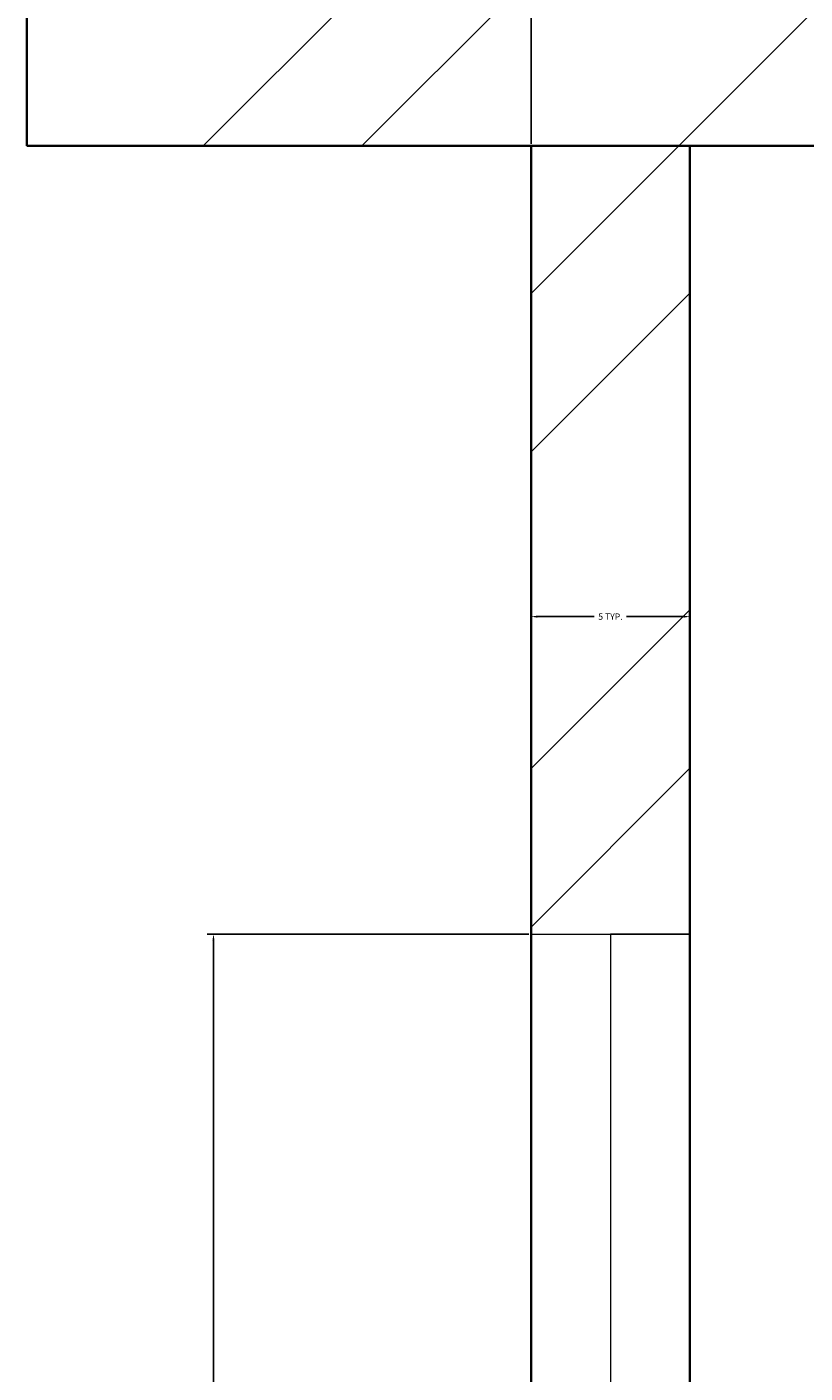
# Model space of a CAD drawing. Units: inches. Extents: x 1962 to 2771, y 1245 to 2660.
# Tile 28 of 114: x 2072 to 2094, y 1894 to 1932. Entities that reach past the tile are written whole.
import ezdxf

# ---------------------------------------------------------------- set-up
doc = ezdxf.new("R2010")
doc.units = ezdxf.units.IN
for name, color, linetype, lineweight in [('A-ANNO-DIMS', 2, 'Continuous', 18), ('A-GLAZ', 4, 'Continuous', 18), ('A-WALL', 7, 'Continuous', 35), ('A-WALL-PATT', 252, 'Continuous', 13)]:
    doc.layers.add(name, color=color, linetype=linetype, lineweight=lineweight)
doc.styles.get("Standard").update_dxf_attribs({"font": 'arial.ttf'})
doc.dimstyles.get("Standard").update_dxf_attribs({"dimtxt": 0.18, "dimasz": 0.18, "dimexe": 0.18, "dimexo": 0.0625, "dimgap": 0.09, "dimtad": 0, "dimtih": 1, "dimtoh": 1, "dimdec": 4, "dimzin": 0, "dimdsep": 46, "dimtxsty": 'Standard', "dimcen": 0.09, "dimadec": 0, "dimazin": 0, "dimtfac": 1, "dimtdec": 4, "dimtofl": 0, "dimtmove": 0, "dimatfit": 3, "dimfxl": 1, "dimtolj": 1, "dimtzin": 0, "dimarcsym": 0})

# ---------------------------------------------------------------- blocks, each defined once
blk = doc.blocks.new('WIN-60IN-A')
for p, q in [((0, 60), (4.5, 60)), ((4.5, 60), (2.25, 60)), ((2.25, 60), (2.25, 0))]:
    blk.add_line(p, q)
blk = doc.blocks.new('*D22')
at = {"layer": 'A-ANNO-DIMS', "color": 0, "lineweight": -2, "transparency": 16777216}
for p, q in [((2086.245, 1906.501), (2077.127, 1906.501)), ((2077.307, 1906.321), (2077.307, 1876.683)), ((2077.307, 1846.681), (2077.307, 1876.319)), ((2086.245, 1846.501), (2077.127, 1846.501))]:
    blk.add_line(p, q, dxfattribs=at)
at = {"layer": 'A-ANNO-DIMS', "color": 0, "transparency": 16777216}
for points in [[(2077.277, 1906.321), (2077.337, 1906.321), (2077.307, 1906.501)], [(2077.277, 1846.681), (2077.337, 1846.681), (2077.307, 1846.501)]]:
    blk.add_solid(points, dxfattribs=at)
at = {"layer": 'Defpoints', "color": 0, "transparency": 16777216}
for p in [(2077.307, 1906.501), (2086.307, 1906.501), (2086.307, 1846.501)]:
    blk.add_point(p, dxfattribs=at)
at = {"layer": 'A-ANNO-DIMS', "color": 0, "transparency": 16777216, "insert": (2077.307, 1876.501), "char_height": 0.18, "attachment_point": 5}
blk.add_mtext('\\A1;W3A 60 TYP.', dxfattribs=at)
blk = doc.blocks.new('*D23')
at = {"layer": 'A-ANNO-DIMS', "color": 0, "lineweight": -2, "transparency": 16777216}
for p, q in [((2086.307, 1906.564), (2086.307, 1915.681)), ((2086.487, 1915.501), (2088.099, 1915.501)), ((2090.627, 1915.501), (2089.016, 1915.501)), ((2090.807, 1906.564), (2090.807, 1915.681))]:
    blk.add_line(p, q, dxfattribs=at)
at = {"layer": 'A-ANNO-DIMS', "color": 0, "transparency": 16777216}
for points in [[(2086.487, 1915.531), (2086.487, 1915.471), (2086.307, 1915.501)], [(2090.627, 1915.531), (2090.627, 1915.471), (2090.807, 1915.501)]]:
    blk.add_solid(points, dxfattribs=at)
at = {"layer": 'Defpoints', "color": 0, "transparency": 16777216}
for p in [(2090.807, 1915.501), (2086.307, 1906.501), (2090.807, 1906.501)]:
    blk.add_point(p, dxfattribs=at)
at = {"layer": 'A-ANNO-DIMS', "color": 0, "transparency": 16777216, "insert": (2088.557, 1915.501), "char_height": 0.18, "attachment_point": 5}
blk.add_mtext('\\A1;5 TYP.', dxfattribs=at)
blk = doc.blocks.new('*D41')
at = {"layer": 'A-ANNO-DIMS', "color": 0, "lineweight": -2, "transparency": 16777216}
for p, q in [((2072.02, 1928.906), (2072.02, 1987.974)), ((2086.307, 1928.906), (2086.307, 1987.974)), ((2072.2, 1987.794), (2078.709, 1987.794)), ((2086.127, 1987.794), (2079.619, 1987.794))]:
    blk.add_line(p, q, dxfattribs=at)
at = {"layer": 'A-ANNO-DIMS', "color": 0, "transparency": 16777216}
for points in [[(2072.2, 1987.824), (2072.2, 1987.764), (2072.02, 1987.794)], [(2086.127, 1987.824), (2086.127, 1987.764), (2086.307, 1987.794)]]:
    blk.add_solid(points, dxfattribs=at)
at = {"layer": 'Defpoints', "color": 0, "transparency": 16777216}
for p in [(2086.307, 1987.794), (2072.02, 1928.844), (2086.307, 1928.844)]:
    blk.add_point(p, dxfattribs=at)
at = {"layer": 'A-ANNO-DIMS', "color": 0, "transparency": 16777216, "insert": (2079.164, 1987.794), "char_height": 0.18, "attachment_point": 5}
blk.add_mtext('\\A1;14.287', dxfattribs=at)

msp = doc.modelspace()

# ---------------------------------------------------------------- hatches: boundary and pattern name
at = {"layer": 'A-WALL-PATT'}
h = msp.add_hatch(dxfattribs=at)
h.set_pattern_fill('ANSI32', color=256)
h.paths.add_polyline_path([(2090.8074, 2467.3437), (2141.6481, 2467.3437), (2141.6481, 2469.5937), (2141.6481, 2471.8437), (2086.3074, 2471.8437), (2086.3074, 2422.5333), (2090.8074, 2422.5333)])
h.paths.add_polyline_path([(2282.7664, 2471.8437), (2204.8982, 2471.8437), (2204.8982, 2467.3437), (2234.8074, 2467.3437), (2234.8074, 2311.3437), (2228.7492, 2311.3437), (2228.7492, 2306.8437), (2234.8074, 2306.8437), (2331.9227, 2306.8437), (2331.9227, 2309.0937), (2331.9227, 2311.3437), (2239.3074, 2311.3437), (2239.3074, 2467.3437), (2282.7664, 2467.3437), (2282.7664, 2469.5937)])
h.paths.add_polyline_path([(2471.4531, 2519.8437), (2552.011, 2519.8437), (2564.3996, 2519.8437), (2564.3996, 2511.1389), (2568.8996, 2511.1389), (2568.8996, 2524.3437), (2466.9531, 2524.3437), (2466.9531, 2471.8437), (2450.0749, 2471.8437), (2446.4672, 2471.8437), (2446.4672, 2467.3437), (2450.0749, 2467.3437), (2475.9988, 2467.3437), (2475.9988, 2469.5937), (2475.9988, 2471.8437), (2471.4531, 2471.8437)])
h.paths.add_polyline_path([(2575.2231, 2469.5937), (2575.2231, 2471.8437), (2568.8996, 2471.8437), (2568.8996, 2487.1389), (2564.3996, 2487.1389), (2564.3996, 2471.8437), (2556.511, 2471.8437), (2499.2904, 2471.8437), (2499.2904, 2467.3437), (2507.8074, 2467.3437), (2507.8074, 2311.3437), (2414.863, 2311.3437), (2414.863, 2306.8437), (2512.3074, 2306.8437), (2517.0114, 2306.8437), (2517.0114, 2309.0937), (2517.0114, 2311.3437), (2512.3074, 2311.3437), (2512.3074, 2467.3437), (2575.2231, 2467.3437)])
h.paths.add_polyline_path([(2660.8074, 2471.8437), (2600.9602, 2471.8437), (2600.9602, 2467.3437), (2656.3074, 2467.3437), (2656.3074, 2432.5704), (2660.8074, 2432.5704)])
h.paths.add_polyline_path([(2660.8074, 2372.5704), (2656.3074, 2372.5704), (2656.3074, 2311.3437), (2600.276, 2311.3437), (2600.276, 2309.0937), (2600.276, 2306.8437), (2656.3074, 2306.8437), (2656.3074, 2296.2593), (2660.8074, 2296.2593)])
h.paths.add_polyline_path([(2572.3074, 2306.8437), (2577.1385, 2306.8437), (2577.1385, 2311.3437), (2551.082, 2311.3437), (2551.082, 2306.8437), (2567.8074, 2306.8437), (2567.8074, 2258.8437), (2540.0574, 2258.8437), (2540.0574, 2256.5937), (2540.0574, 2254.3437), (2567.8074, 2254.3437), (2656.3074, 2254.3437), (2656.3074, 2236.9085), (2660.8074, 2236.9085), (2660.8074, 2272.2593), (2656.3074, 2272.2593), (2656.3074, 2258.8437), (2572.3074, 2258.8437)])
h.paths.add_polyline_path([(2512.3074, 2254.3437), (2518.8716, 2254.3437), (2518.8716, 2256.5937), (2518.8716, 2258.8437), (2507.8074, 2258.8437), (2507.8074, 2177.8437), (2567.8074, 2177.8437), (2567.8074, 2172.9628), (2572.3074, 2172.9628), (2572.3074, 2177.8437), (2656.3074, 2177.8437), (2656.3074, 2166.4846), (2660.8074, 2166.4846), (2660.8074, 2200.9085), (2656.3074, 2200.9085), (2656.3074, 2182.3437), (2512.3074, 2182.3437)])
h.paths.add_polyline_path([(2656.3074, 2129.8437), (2572.3074, 2129.8437), (2572.3074, 2150.3044), (2570.0574, 2150.3044), (2567.8074, 2150.3044), (2567.8074, 2129.8437), (2507.8074, 2129.8437), (2507.8074, 2116.3027), (2510.0574, 2116.3027), (2512.3074, 2116.3027), (2512.3074, 2125.3437), (2567.8074, 2125.3437), (2572.3074, 2125.3437), (2656.3074, 2125.3437)])
h.paths.add_polyline_path([(2090.8074, 2362.5333), (2086.3074, 2362.5333), (2086.3074, 2298.6242), (2090.8074, 2298.6242), (2090.8074, 2306.8437), (2174.8074, 2306.8437), (2174.8074, 2286.4178), (2179.3074, 2286.4178), (2179.3074, 2306.8437), (2192.8641, 2306.8437), (2192.8641, 2309.0937), (2192.8641, 2311.3437), (2090.8074, 2311.3437)])
h.paths.add_polyline_path([(2209.156, 2258.8437), (2179.3074, 2258.8437), (2179.3074, 2263.2236), (2177.0574, 2263.2236), (2174.8074, 2263.2236), (2174.8074, 2258.8437), (2090.8074, 2258.8437), (2090.8074, 2274.6242), (2086.3074, 2274.6242), (2086.3074, 2238.2967), (2088.5574, 2238.2967), (2090.8074, 2238.2967), (2090.8074, 2254.3437), (2209.156, 2254.3437)])
h.paths.add_polyline_path([(2090.8074, 2177.8437), (2234.8074, 2177.8437), (2234.8074, 2173.1428), (2239.3074, 2173.1428), (2239.3074, 2258.8437), (2230.8442, 2258.8437), (2230.8442, 2256.5937), (2230.8442, 2254.3437), (2234.8074, 2254.3437), (2234.8074, 2182.3437), (2090.8074, 2182.3437), (2090.8074, 2202.2967), (2086.3074, 2202.2967), (2086.3074, 2140.0389), (2090.8074, 2140.0389)])
h.paths.add_polyline_path([(2090.8074, 2080.0389), (2086.3074, 2080.0389), (2086.3074, 2033.8437), (2090.8074, 2033.8437)], flags=17)
h.paths.add_polyline_path([(2244.9405, 2033.8437), (2239.3074, 2033.8437), (2239.3074, 2142.0665), (2237.2592, 2142.0665), (2234.8074, 2142.0665), (2234.8074, 2033.8437), (2090.8074, 2033.8437), (2076.5204, 2033.8437), (2072.0204, 2033.8437), (2072.0204, 2000.4493), (2076.5204, 2000.4493), (2076.5204, 2029.3437), (2090.8074, 2029.3437), (2244.9405, 2029.3437), (2244.9405, 2031.5937)])
h.paths.add_polyline_path([(2234.8074, 1933.3437), (2076.5204, 1933.3437), (2076.5204, 1952.4493), (2074.2704, 1952.4493), (2072.0204, 1952.4493), (2072.0204, 1933.3437), (2072.0204, 1928.8437), (2234.8074, 1928.8437)])
h.paths.add_polyline_path([(2090.8074, 1928.8437), (2086.3074, 1928.8437), (2086.3074, 1906.5013), (2090.8074, 1906.5013)])
h.paths.add_polyline_path([(2090.8074, 1846.5013), (2086.3074, 1846.5013), (2086.3074, 1769.9917), (2088.5574, 1769.9917), (2090.8074, 1769.9917), (2090.8074, 1780.3437), (2234.8074, 1780.3437), (2234.8074, 1708.3437), (2230.3764, 1708.3437), (2230.3764, 1703.8437), (2239.3074, 1703.8437), (2239.3074, 1792.6669), (2237.0574, 1792.6669), (2234.8074, 1792.6669), (2234.8074, 1784.8437), (2090.8074, 1784.8437)])
h.paths.add_polyline_path([(2239.3074, 1928.8437), (2244.9405, 1928.8437), (2244.9405, 1931.0937), (2244.9405, 1933.3437), (2234.8074, 1933.3437), (2234.8074, 1928.8437), (2234.8074, 1825.5949), (2239.3074, 1825.5949)])
h.paths.add_polyline_path([(2148.0425, 1649.0937), (2148.0425, 1651.3437), (2090.8074, 1651.3437), (2090.8074, 1646.8437), (2148.0425, 1646.8437)], flags=0)
h.paths.add_polyline_path([(2207.5601, 1708.3437), (2090.8074, 1708.3437), (2090.8074, 1703.8437), (2174.8074, 1703.8437), (2174.8074, 1651.3437), (2170.4457, 1651.3437), (2170.4457, 1646.8437), (2195.9924, 1646.8437), (2195.9924, 1649.0937), (2195.9924, 1651.3437), (2179.3074, 1651.3437), (2179.3074, 1703.8437), (2207.5601, 1703.8437), (2207.5601, 1706.0937)])
h.paths.add_polyline_path([(2090.8074, 1733.9917), (2086.3074, 1733.9917), (2086.3074, 1696.1032), (2088.5574, 1696.1032), (2090.8074, 1696.1032)])
h.paths.add_polyline_path([(2090.8074, 1672.1032), (2086.3074, 1672.1032), (2086.3074, 1600.3335), (2090.8074, 1600.3335)])
h.paths.add_polyline_path([(2090.8074, 1540.3335), (2086.3074, 1540.3335), (2086.3074, 1486.3437), (2139.6766, 1486.3437), (2139.6766, 1490.8437), (2090.8074, 1490.8437)])
h.paths.add_polyline_path([(2302.3876, 1490.8437), (2239.3074, 1490.8437), (2239.3074, 1646.8437), (2335.9994, 1646.8437), (2335.9994, 1651.3437), (2229.884, 1651.3437), (2229.884, 1646.8437), (2234.8074, 1646.8437), (2234.8074, 1490.8437), (2202.7103, 1490.8437), (2202.7103, 1488.5937), (2202.7103, 1486.3437), (2275.0699, 1486.3437), (2275.0699, 1475.772), (2279.5699, 1475.772), (2279.5699, 1486.3437), (2302.3876, 1486.3437)])
h.paths.add_polyline_path([(2279.5699, 1451.772), (2275.0699, 1451.772), (2275.0699, 1438.3437), (2174.8074, 1438.3437), (2174.8074, 1486.3437), (2179.7922, 1486.3437), (2179.7922, 1490.8437), (2163.3585, 1490.8437), (2163.3585, 1488.5937), (2163.3585, 1486.3437), (2170.3074, 1486.3437), (2170.3074, 1433.8437), (2279.5699, 1433.8437)])
h.paths.add_polyline_path([(2427.2363, 1490.8437), (2375.8074, 1490.8437), (2375.8074, 1646.8437), (2381.6401, 1646.8437), (2381.6401, 1651.3437), (2365.887, 1651.3437), (2365.887, 1649.0937), (2365.887, 1646.8437), (2371.3074, 1646.8437), (2371.3074, 1490.8437), (2327.5627, 1490.8437), (2327.5627, 1488.5937), (2327.5627, 1486.3437), (2371.3074, 1486.3437), (2371.3074, 1433.8437), (2375.8074, 1433.8437), (2375.8074, 1486.3437), (2427.2363, 1486.3437)])
h.paths.add_polyline_path([(2512.3074, 1646.8437), (2519.4351, 1646.8437), (2519.4351, 1649.0937), (2519.4351, 1651.3437), (2507.8074, 1651.3437), (2416.0063, 1651.3437), (2416.0063, 1649.0937), (2416.0063, 1646.8437), (2507.8074, 1646.8437), (2507.8074, 1490.8437), (2497.0532, 1490.8437), (2497.0532, 1488.5937), (2497.0532, 1486.3437), (2574.9344, 1486.3437), (2574.9344, 1476.0181), (2579.4344, 1476.0181), (2579.4344, 1486.3437), (2584.4872, 1486.3437), (2584.3074, 1490.8437), (2512.3074, 1490.8437)])
h.paths.add_polyline_path([(2470.5091, 1486.3437), (2473.9767, 1486.3437), (2473.9767, 1490.8437), (2449.6605, 1490.8437), (2449.6605, 1488.5937), (2449.6605, 1486.3437), (2466.0091, 1486.3437), (2466.0091, 1433.8437), (2470.5091, 1433.8437), (2579.4344, 1433.8437), (2579.4344, 1452.0181), (2574.9344, 1452.0181), (2574.9344, 1438.3437), (2554.5091, 1438.3437), (2470.5091, 1438.3437)])
h.paths.add_polyline_path([(2656.3074, 1490.8437), (2611.86, 1490.8437), (2611.86, 1486.3437), (2656.3074, 1486.3437)])
h.paths.add_polyline_path([(2660.8074, 1532.7007), (2658.5574, 1532.7007), (2656.3074, 1532.7007), (2656.3074, 1486.3437), (2660.8074, 1486.3437)])
h.paths.add_polyline_path([(2660.8074, 1664.9663), (2656.3074, 1664.9663), (2656.3074, 1651.3437), (2602.2313, 1651.3437), (2602.2313, 1646.8437), (2656.3074, 1646.8437), (2656.3074, 1592.7007), (2660.8074, 1592.7007)])
h.paths.add_polyline_path([(2660.8074, 1724.5221), (2656.3074, 1724.5221), (2656.3074, 1703.8437), (2542.4725, 1703.8437), (2542.4725, 1699.3437), (2567.8074, 1699.3437), (2567.8074, 1651.3437), (2552.7766, 1651.3437), (2552.7766, 1649.0937), (2552.7766, 1646.8437), (2577.2878, 1646.8437), (2577.2878, 1649.0937), (2577.2878, 1651.3437), (2572.3074, 1651.3437), (2572.3074, 1699.3437), (2656.3074, 1699.3437), (2656.3074, 1688.9663), (2660.8074, 1688.9663)])
h.paths.add_polyline_path([(2660.8074, 1880.6524), (2656.3074, 1880.6524), (2656.3074, 1832.8437), (2512.3074, 1832.8437), (2512.3074, 1837.8959), (2507.8074, 1837.8959), (2507.8074, 1828.3437), (2567.8074, 1828.3437), (2567.8074, 1804.3437), (2572.3074, 1804.3437), (2572.3074, 1828.3437), (2656.3074, 1828.3437), (2656.3074, 1818.6778), (2660.8074, 1818.6778)])
h.paths.add_polyline_path([(2660.8074, 1794.6778), (2656.3074, 1794.6778), (2656.3074, 1780.3437), (2572.3074, 1780.3437), (2572.3074, 1783.0303), (2570.0574, 1783.0303), (2567.8074, 1783.0303), (2567.8074, 1780.3437), (2507.8074, 1780.3437), (2507.8074, 1699.3437), (2517.8858, 1699.3437), (2517.8858, 1701.5937), (2517.8858, 1703.8437), (2512.3074, 1703.8437), (2512.3074, 1775.8437), (2656.3074, 1775.8437), (2656.3074, 1760.5221), (2660.8074, 1760.5221)])
h.paths.add_polyline_path([(2660.8074, 1981.3437), (2660.8074, 2020.2808), (2658.5574, 2020.2808), (2656.3074, 2020.2808), (2656.3074, 1981.3437), (2512.3074, 1981.3437), (2512.3074, 2086.6996), (2507.8074, 2086.6996), (2507.8074, 1981.3437), (2375.8074, 1981.3437), (2375.8074, 1986.8505), (2373.5574, 1986.8505), (2371.3074, 1986.8505), (2371.3074, 1973.2607), (2375.8074, 1973.2607), (2375.8074, 1976.8437), (2507.8074, 1976.8437), (2507.8074, 1865.4281), (2510.0574, 1865.4281), (2512.3074, 1865.4281), (2512.3074, 1976.8437), (2660.8074, 1976.8437)])
h.paths.add_polyline_path([(2375.8074, 1940.297), (2373.5574, 1940.297), (2371.3074, 1940.297), (2371.3074, 1933.3437), (2278.4434, 1933.3437), (2278.4434, 1928.8437), (2371.3074, 1928.8437), (2371.3074, 1651.3437), (2375.8074, 1651.3437)])
h.paths.add_polyline_path([(2660.8074, 1976.8437), (2656.3074, 1976.8437), (2656.3074, 1940.6524), (2660.8074, 1940.6524)], flags=17)
h.paths.add_polyline_path([(2660.8074, 2142.4846), (2656.3074, 2142.4846), (2656.3074, 2080.2808), (2660.8074, 2080.2808)])
h.paths.add_polyline_path([(2381.4189, 2311.3437), (2375.8074, 2311.3437), (2375.8074, 2467.3437), (2424.7242, 2467.3437), (2424.7242, 2469.5937), (2424.7242, 2471.8437), (2375.8074, 2471.8437), (2375.8074, 2524.3437), (2371.3074, 2524.3437), (2371.3074, 2471.8437), (2307.2097, 2471.8437), (2307.2097, 2467.3437), (2371.3074, 2467.3437), (2371.3074, 2311.3437), (2366.8901, 2311.3437), (2366.8901, 2306.8437), (2371.3074, 2306.8437), (2371.3074, 2033.8437), (2279.6589, 2033.8437), (2279.6589, 2029.3437), (2371.3074, 2029.3437), (2371.3074, 2014.2598), (2375.8074, 2014.2598), (2375.8074, 2306.8437), (2381.4189, 2306.8437)])
h.paths.add_polyline_path([(2263.3074, 2524.3437), (2170.3074, 2524.3437), (2170.3074, 2519.8437), (2170.3074, 2471.8437), (2165.0312, 2471.8437), (2165.0312, 2467.3437), (2179.6721, 2467.3437), (2179.6721, 2469.5161), (2179.6721, 2471.8437), (2174.8074, 2471.8437), (2174.8074, 2519.8437), (2258.8074, 2519.8437), (2258.8074, 2511.6436), (2263.3074, 2511.6436)])
h.paths.add_polyline_path([(2245.0232, 1361.4123), (2492.9468, 1361.4123), (2492.9468, 1398.505), (2245.0232, 1398.505)], flags=9)
h.paths.add_polyline_path([(2388.1434, 2086.6936), (2425.0704, 2086.6936), (2425.0704, 2105.3509), (2388.1434, 2105.3509)], flags=9)
h.paths.add_polyline_path([(2404.922, 2242.6744), (2445.7337, 2242.6744), (2445.7337, 2261.3318), (2404.922, 2261.3318)], flags=9)
h.paths.add_polyline_path([(2269.4107, 2156.7935), (2306.3378, 2156.7935), (2306.3378, 2175.4508), (2269.4107, 2175.4508)], flags=9)
h.paths.add_polyline_path([(2269.3277, 2233.4343), (2306.2547, 2233.4343), (2306.2547, 2252.0917), (2269.3277, 2252.0917)], flags=9)
h.paths.add_polyline_path([(2431.6052, 2320.6922), (2470.4456, 2320.6922), (2470.4456, 2339.3495), (2431.6052, 2339.3495)], flags=25)
h.paths.add_polyline_path([(2249.6902, 2315.7608), (2288.5306, 2315.7608), (2288.5306, 2334.4182), (2249.6902, 2334.4182)], flags=25)
h.paths.add_polyline_path([(2096.9301, 2314.3181), (2135.7704, 2314.3181), (2135.7704, 2332.9755), (2096.9301, 2332.9755)], flags=25)
h.paths.add_polyline_path([(2134.3475, 2285.7089), (2161.4655, 2285.7089), (2161.4655, 2304.3662), (2134.3475, 2304.3662)], flags=9)
h.paths.add_polyline_path([(2126.5155, 2209.4076), (2159.9227, 2209.4076), (2159.9227, 2228.065), (2126.5155, 2228.065)], flags=25)
h.paths.add_polyline_path([(2110.5753, 2141.5299), (2149.4157, 2141.5299), (2149.4157, 2160.1872), (2110.5753, 2160.1872)], flags=25)
h.paths.add_polyline_path([(2249.8618, 1968.3317), (2286.3966, 1968.3317), (2286.3966, 1986.989), (2249.8618, 1986.989)], flags=9)
h.paths.add_polyline_path([(2395.9507, 1777.0051), (2436.7624, 1777.0051), (2436.7624, 1795.6625), (2395.9507, 1795.6625)], flags=9)
h.paths.add_polyline_path([(2398.5259, 1888.5651), (2435.0062, 1888.5651), (2435.0062, 1907.2224), (2398.5259, 1907.2224)], flags=25)
h.paths.add_polyline_path([(2259.3506, 1728.3559), (2296.2776, 1728.3559), (2296.2776, 1747.0132), (2259.3506, 1747.0132)], flags=9)
h.paths.add_polyline_path([(2271.3698, 1845.268), (2308.2968, 1845.268), (2308.2968, 1863.9253), (2271.3698, 1863.9253)], flags=9)
h.paths.add_polyline_path([(2120.9355, 1786.3027), (2159.7759, 1786.3027), (2159.7759, 1804.9601), (2120.9355, 1804.9601)], flags=25)
h.paths.add_polyline_path([(2121.3164, 1732.1043), (2154.7236, 1732.1043), (2154.7236, 1750.7616), (2121.3164, 1750.7616)], flags=25)
h.paths.add_polyline_path([(2118.3706, 1678.8997), (2147.5282, 1678.8997), (2147.5282, 1697.557), (2118.3706, 1697.557)], flags=25)
h.paths.add_polyline_path([(2385.9227, 1493.557), (2424.763, 1493.557), (2424.763, 1512.2143), (2385.9227, 1512.2143)], flags=25)
h.paths.add_polyline_path([(2248.7058, 1500.0256), (2287.5462, 1500.0256), (2287.5462, 1518.6829), (2248.7058, 1518.6829)], flags=25)
h.paths.add_polyline_path([(2104.1669, 1617.3771), (2143.0073, 1617.3771), (2143.0073, 1636.0344), (2104.1669, 1636.0344)], flags=9)
h.paths.add_polyline_path([(2096.0714, 1447.8824), (2137.3845, 1447.8824), (2137.3845, 1458.1859), (2096.0714, 1458.1859)], flags=9)
h.paths.add_polyline_path([(2180.6114, 1440.325), (2209.7689, 1440.325), (2209.7689, 1458.9823), (2180.6114, 1458.9823)], flags=25)
h.paths.add_polyline_path([(2316.1698, 1447.9637), (2357.4829, 1447.9637), (2357.4829, 1458.2673), (2316.1698, 1458.2673)], flags=9)
h.paths.add_polyline_path([(2397.6187, 1447.9637), (2438.9318, 1447.9637), (2438.9318, 1458.2673), (2397.6187, 1458.2673)], flags=9)
h.paths.add_polyline_path([(2473.0778, 1439.5953), (2502.2354, 1439.5953), (2502.2354, 1458.2527), (2473.0778, 1458.2527)], flags=25)
h.paths.add_polyline_path([(2589.7027, 1447.8819), (2631.0158, 1447.8819), (2631.0158, 1458.1855), (2589.7027, 1458.1855)], flags=9)
h.paths.add_polyline_path([(2522.4009, 1497.5285), (2561.2413, 1497.5285), (2561.2413, 1516.1859), (2522.4009, 1516.1859)], flags=25)
h.paths.add_polyline_path([(2579.6565, 1671.3482), (2608.8141, 1671.3482), (2608.8141, 1690.0056), (2579.6565, 1690.0056)], flags=25)
h.paths.add_polyline_path([(2544.7038, 1725.5064), (2578.1111, 1725.5064), (2578.1111, 1744.1637), (2544.7038, 1744.1637)], flags=25)
h.paths.add_polyline_path([(2578.1191, 1807.472), (2607.2766, 1807.472), (2607.2766, 1826.1293), (2578.1191, 1826.1293)], flags=25)
h.paths.add_polyline_path([(2595.0614, 1835.1839), (2633.9018, 1835.1839), (2633.9018, 1853.8413), (2595.0614, 1853.8413)], flags=25)
h.paths.add_polyline_path([(2567.0097, 2097.7035), (2605.8501, 2097.7035), (2605.8501, 2116.3609), (2567.0097, 2116.3609)], flags=9)
h.paths.add_polyline_path([(2586.644, 2134.6454), (2615.8015, 2134.6454), (2615.8015, 2153.3027), (2586.644, 2153.3027)], flags=9)
h.paths.add_polyline_path([(2544.6185, 2212.6783), (2578.0258, 2212.6783), (2578.0258, 2231.3356), (2544.6185, 2231.3356)], flags=25)
h.paths.add_polyline_path([(2577.0273, 2256.9023), (2606.1849, 2256.9023), (2606.1849, 2275.5597), (2577.0273, 2275.5597)], flags=24)
h.paths.add_polyline_path([(2605.2683, 2315.2821), (2644.1087, 2315.2821), (2644.1087, 2333.9395), (2605.2683, 2333.9395)], flags=25)
h.paths.add_polyline_path([(2583.1244, 2496.1815), (2624.4375, 2496.1815), (2624.4375, 2506.4851), (2583.1244, 2506.4851)], flags=9)
h.paths.add_polyline_path([(2474.761, 2497.0823), (2503.9185, 2497.0823), (2503.9185, 2515.7397), (2474.761, 2515.7397)], flags=25)
h.paths.add_polyline_path([(2387.5787, 2494.2563), (2428.902, 2494.2563), (2428.902, 2504.5598), (2387.5787, 2504.5598)], flags=9)
h.paths.add_polyline_path([(2300.1657, 2500.1564), (2341.4788, 2500.1564), (2341.4788, 2510.46), (2300.1657, 2510.46)], flags=25)
h.paths.add_polyline_path([(2176.8589, 2497.5843), (2206.0165, 2497.5843), (2206.0165, 2516.2416), (2176.8589, 2516.2416)], flags=25)
h.paths.add_polyline_path([(2097.4668, 2494.9762), (2138.7799, 2494.9762), (2138.7799, 2505.2798), (2097.4668, 2505.2798)], flags=9)

# ---------------------------------------------------------------- linework, layer by layer
at = {"layer": 'A-WALL'}
for p, q in [((2072.0204, 1933.3437), (2072.0204, 1928.8437)), ((2072.0204, 1928.8437), (2234.8074, 1928.8437)), ((2086.3074, 1928.8437), (2086.3074, 1486.3437)), ((2090.8074, 1928.8437), (2090.8074, 1784.8437))]:
    msp.add_line(p, q, dxfattribs=at)

# ---------------------------------------------------------------- block references
at = {"layer": 'A-GLAZ'}
msp.add_blockref('WIN-60IN-A', (2086.3074, 1846.5013), dxfattribs=at)

# ---------------------------------------------------------------- dimensions: what is measured, and where the dimension line sits
at = {"layer": 'A-ANNO-DIMS'}
dim = msp.add_linear_dim(base=(2086.3074, 1987.7937), p1=(2072.0204, 1928.8437), p2=(2086.3074, 1928.8437), dimstyle='Standard', override={"dimdec": 3, "dimlfac": 1, "dimrnd": 0, "dimzin": 0, "dimdsep": 46, "dimlunit": 2}, dxfattribs=at)
dim.commit()
dim.dimension.update_dxf_attribs({"geometry": '*D41', "text_midpoint": (2079.1639, 1987.7937)})
dim = msp.add_linear_dim(base=(2090.8073805882, 1915.5012743401), p1=(2086.3073805882, 1906.5012743401), p2=(2090.8073805882, 1906.5012743401), text='<> TYP.', dimstyle='Standard', override={"dimdec": 0, "dimlfac": 1, "dimrnd": 0, "dimzin": 0, "dimdsep": 46, "dimlunit": 2}, dxfattribs=at)
dim.commit()
dim.dimension.update_dxf_attribs({"geometry": '*D23', "text_midpoint": (2088.5573805882, 1915.5012743401)})
dim = msp.add_linear_dim(base=(2077.3074, 1906.5013), p1=(2086.3074, 1846.5013), p2=(2086.3074, 1906.5013), angle=90, text='W3A <> TYP.', dimstyle='Standard', override={"dimdec": 0, "dimlfac": 1, "dimrnd": 0, "dimzin": 0, "dimdsep": 46, "dimlunit": 2}, dxfattribs=at)
dim.commit()
dim.dimension.update_dxf_attribs({"geometry": '*D22', "text_midpoint": (2077.3074, 1876.5013)})

doc.saveas('drawing.dxf')
